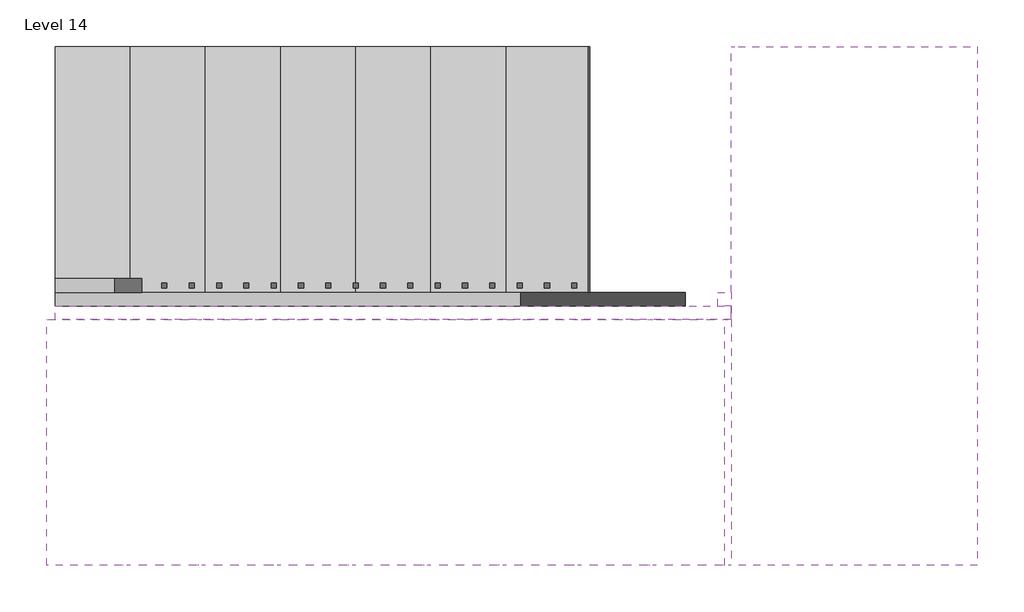
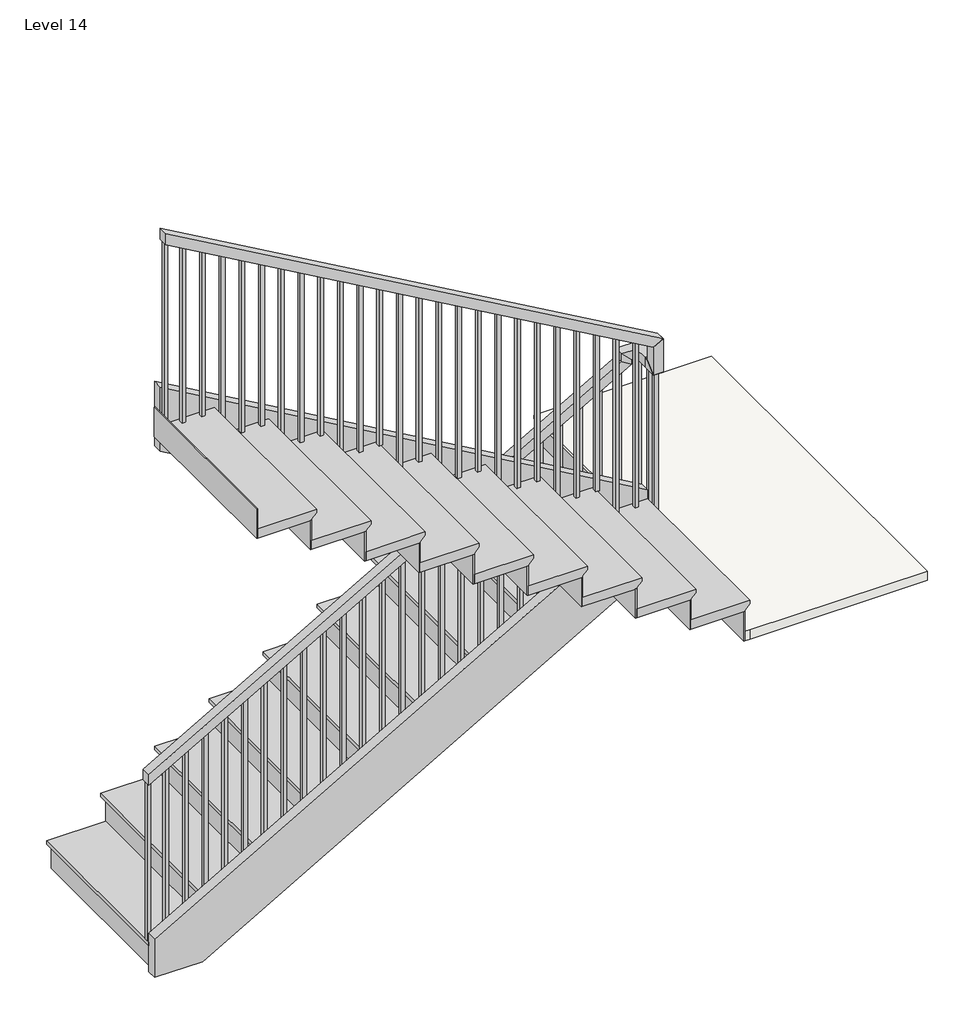
# One storey: 3 members, 2 stair flights, 1 railing, 1 slab.
"""IFC4 building model written with IfcOpenShell, lengths in millimetres."""

from ifc_helpers import new_model, si_unit, frame, origin, place, context, project, spatial, polyline, outline, extrude, faceted_brep, transform, mapped, element, save
from components import non_monolithic_landing_f7b8efd9, stair_flight_4ab4d81b, stair_flight_a571a0bd

model = new_model("IFC4")

# Units and contexts
model_context = context("Model", 3, world=origin())
ifc_project = project(units=[si_unit("LENGTHUNIT", "METRE", prefix="MILLI")], contexts=[model_context])

# Site, building, storey
site = spatial("IfcSite", under=ifc_project)
building = spatial("IfcBuilding", under=site)
storey = spatial("IfcBuildingStorey", under=building, Name="Level 14", Elevation=6400.8)

# Members
placement = place(None, origin())
element("IfcMember", 1, ObjectType="Stringer - 2\" Width", at=placement, inside=storey, context=model_context, shape_type="SweptSolid", body=[
    extrude(outline(polyline([(6609.8890626, -1591.1154463), (6400.8, -1591.1154463), (6400.8, -1342.8974141), (7669.724218, 872.6845537), (8020.9745172, 872.6845537), (6609.8890626, -1591.1154463)])), frame((0.0, -4788.1544725, 0.0), z_axis=(0.0, 1.0, 0.0), x_axis=(0.0, 0.0, 1.0)), (0.0, 0.0, 1.0), 50.8),
])
element("IfcMember", 2, ObjectType="Stringer - 2\" Width", at=placement, inside=storey, context=model_context, shape_type="SweptSolid", body=[
    extrude(outline(polyline([(7858.8387634, 923.4845537), (8210.0890626, 923.4845537), (9650.2690626, -1591.1154463), (9299.0187634, -1591.1154463), (7858.8387634, 923.4845537)])), frame((0.0, -4838.9544725, 0.0), z_axis=(0.0, 1.0, 0.0), x_axis=(0.0, 0.0, 1.0)), (0.0, 0.0, 1.0), 50.8),
])
element("IfcMember", 3, ObjectType="Stringer - 2\" Width", at=placement, inside=storey, context=model_context, shape_type="SweptSolid", body=[
    extrude(outline(polyline([(872.6845537, -4737.3544725), (923.4845537, -4737.3544725), (923.4845537, -4788.1544725), (872.6845537, -4788.1544725), (872.6845537, -4737.3544725)])), frame((0.0, 0.0, 7772.4), z_axis=(0.0, 0.0, 1.0), x_axis=(1.0, 0.0, 0.0)), (0.0, 0.0, 1.0), 304.8),
])

# Railing
element("IfcRailing", 4, ObjectType="Handrail - Rectangular", at=placement, inside=storey, context=model_context, shape_type="SolidModel", body=[
    faceted_brep([(-1591.1154463, -4686.5544725, 7475.22), (-1591.1154463, -4686.5544725, 7416.6782835), (-1591.1154463, -4737.3544725, 7416.6782835), (-1591.1154463, -4737.3544725, 7475.22), (847.2845537, -4686.5544725, 8871.7581818), (898.0845537, -4686.5544725, 8842.3110107), (898.0845537, -4737.3544725, 8842.3110107), (847.2845537, -4737.3544725, 8871.7581818), (847.2845537, -4686.5544725, 8915.4), (898.0845537, -4686.5544725, 8864.6), (898.0845537, -4737.3544725, 8864.6), (847.2845537, -4737.3544725, 8915.4), (974.2845537, -4686.5544725, 8915.4), (974.2845537, -4686.5544725, 8864.6), (923.4845537, -4737.3544725, 8864.6), (923.4845537, -4737.3544725, 8915.4), (974.2845537, -4813.5544725, 8915.4), (974.2845537, -4813.5544725, 8864.6), (923.4845537, -4813.5544725, 8864.6), (923.4845537, -4813.5544725, 8915.4), (974.2845537, -4838.9544725, 8915.4), (923.4845537, -4838.9544725, 8915.4), (923.4845537, -4889.7544725, 8864.6), (974.2845537, -4889.7544725, 8864.6)], [[[0, 1, 2, 3]], [[1, 0, 4, 5]], [[2, 1, 5, 6]], [[3, 2, 6, 7]], [[0, 3, 7, 4]], [[5, 4, 8, 9]], [[6, 5, 9, 10]], [[7, 6, 10, 11]], [[4, 7, 11, 8]], [[9, 8, 12, 13]], [[10, 9, 13, 14]], [[11, 10, 14, 15]], [[8, 11, 15, 12]], [[13, 12, 16, 17]], [[14, 13, 17, 18]], [[15, 14, 18, 19]], [[12, 15, 19, 16]], [[20, 21, 22, 23]], [[17, 16, 20, 23]], [[18, 17, 23, 22]], [[19, 18, 22, 21]], [[16, 19, 21, 20]]]),
    faceted_brep([(974.2845537, -4838.9544725, 8915.4), (974.2845537, -4889.7544725, 8864.6), (923.4845537, -4889.7544725, 8864.6), (923.4845537, -4838.9544725, 8915.4), (974.2845537, -4838.9544725, 9046.3254545), (923.4845537, -4838.9544725, 9016.8782835), (923.4845537, -4889.7544725, 9016.8782835), (974.2845537, -4889.7544725, 9046.3254545)], [[[0, 1, 2, 3]], [[4, 5, 6, 7]], [[1, 0, 4, 7]], [[2, 1, 7, 6]], [[3, 2, 6, 5]], [[0, 3, 5, 4]]]),
    faceted_brep([(974.2845537, -4889.7544725, 9046.3254545), (923.4845537, -4889.7544725, 9016.8782835), (923.4845537, -4838.9544725, 9016.8782835), (974.2845537, -4838.9544725, 9046.3254545), (-1591.1154463, -4889.7544725, 10515.6), (-1591.1154463, -4838.9544725, 10515.6), (-1591.1154463, -4838.9544725, 10457.0582835), (-1591.1154463, -4889.7544725, 10457.0582835)], [[[0, 1, 2, 3]], [[4, 5, 6, 7]], [[1, 0, 4, 7]], [[2, 1, 7, 6]], [[3, 2, 6, 5]], [[0, 3, 5, 4]]]),
    extrude(outline(polyline([(10393.4139653, -1479.9904463), (10404.3244198, -1499.0404463), (9441.18, -1499.0404463), (9441.18, -1479.9904463), (10393.4139653, -1479.9904463)])), frame((0.0, -4873.8794725, 0.0), z_axis=(0.0, 1.0, 0.0), x_axis=(0.0, 0.0, 1.0)), (0.0, 0.0, 1.0), 19.05),
    extrude(outline(polyline([(10335.2248744, -1378.3904463), (10346.1353289, -1397.4404463), (9441.18, -1397.4404463), (9441.18, -1378.3904463), (10335.2248744, -1378.3904463)])), frame((0.0, -4873.8794725, 0.0), z_axis=(0.0, 1.0, 0.0), x_axis=(0.0, 0.0, 1.0)), (0.0, 0.0, 1.0), 19.05),
    extrude(outline(polyline([(10277.0357835, -1276.7904463), (10287.946238, -1295.8404463), (9281.16, -1295.8404463), (9281.16, -1276.7904463), (10277.0357835, -1276.7904463)])), frame((0.0, -4873.8794725, 0.0), z_axis=(0.0, 1.0, 0.0), x_axis=(0.0, 0.0, 1.0)), (0.0, 0.0, 1.0), 19.05),
    extrude(outline(polyline([(10218.8466926, -1175.1904463), (10229.7571471, -1194.2404463), (9281.16, -1194.2404463), (9281.16, -1175.1904463), (10218.8466926, -1175.1904463)])), frame((0.0, -4873.8794725, 0.0), z_axis=(0.0, 1.0, 0.0), x_axis=(0.0, 0.0, 1.0)), (0.0, 0.0, 1.0), 19.05),
    extrude(outline(polyline([(10160.6576016, -1073.5904463), (10171.5680562, -1092.6404463), (9281.16, -1092.6404463), (9281.16, -1073.5904463), (10160.6576016, -1073.5904463)])), frame((0.0, -4873.8794725, 0.0), z_axis=(0.0, 1.0, 0.0), x_axis=(0.0, 0.0, 1.0)), (0.0, 0.0, 1.0), 19.05),
    extrude(outline(polyline([(10102.4685107, -971.9904463), (10113.3789653, -991.0404463), (9121.14, -991.0404463), (9121.14, -971.9904463), (10102.4685107, -971.9904463)])), frame((0.0, -4873.8794725, 0.0), z_axis=(0.0, 1.0, 0.0), x_axis=(0.0, 0.0, 1.0)), (0.0, 0.0, 1.0), 19.05),
    extrude(outline(polyline([(10044.2794198, -870.3904463), (10055.1898744, -889.4404463), (9121.14, -889.4404463), (9121.14, -870.3904463), (10044.2794198, -870.3904463)])), frame((0.0, -4873.8794725, 0.0), z_axis=(0.0, 1.0, 0.0), x_axis=(0.0, 0.0, 1.0)), (0.0, 0.0, 1.0), 19.05),
    extrude(outline(polyline([(9986.0903289, -768.7904463), (9997.0007835, -787.8404463), (9121.14, -787.8404463), (9121.14, -768.7904463), (9986.0903289, -768.7904463)])), frame((0.0, -4873.8794725, 0.0), z_axis=(0.0, 1.0, 0.0), x_axis=(0.0, 0.0, 1.0)), (0.0, 0.0, 1.0), 19.05),
    extrude(outline(polyline([(9927.901238, -667.1904463), (9938.8116926, -686.2404463), (8961.12, -686.2404463), (8961.12, -667.1904463), (9927.901238, -667.1904463)])), frame((0.0, -4873.8794725, 0.0), z_axis=(0.0, 1.0, 0.0), x_axis=(0.0, 0.0, 1.0)), (0.0, 0.0, 1.0), 19.05),
    extrude(outline(polyline([(9869.7121471, -565.5904463), (9880.6226016, -584.6404463), (8961.12, -584.6404463), (8961.12, -565.5904463), (9869.7121471, -565.5904463)])), frame((0.0, -4873.8794725, 0.0), z_axis=(0.0, 1.0, 0.0), x_axis=(0.0, 0.0, 1.0)), (0.0, 0.0, 1.0), 19.05),
    extrude(outline(polyline([(9811.5230562, -463.9904463), (9822.4335107, -483.0404463), (8961.12, -483.0404463), (8961.12, -463.9904463), (9811.5230562, -463.9904463)])), frame((0.0, -4873.8794725, 0.0), z_axis=(0.0, 1.0, 0.0), x_axis=(0.0, 0.0, 1.0)), (0.0, 0.0, 1.0), 19.05),
    extrude(outline(polyline([(9753.3339653, -362.3904463), (9764.2444198, -381.4404463), (8801.1, -381.4404463), (8801.1, -362.3904463), (9753.3339653, -362.3904463)])), frame((0.0, -4873.8794725, 0.0), z_axis=(0.0, 1.0, 0.0), x_axis=(0.0, 0.0, 1.0)), (0.0, 0.0, 1.0), 19.05),
    extrude(outline(polyline([(9695.1448744, -260.7904463), (9706.0553289, -279.8404463), (8801.1, -279.8404463), (8801.1, -260.7904463), (9695.1448744, -260.7904463)])), frame((0.0, -4873.8794725, 0.0), z_axis=(0.0, 1.0, 0.0), x_axis=(0.0, 0.0, 1.0)), (0.0, 0.0, 1.0), 19.05),
    extrude(outline(polyline([(9636.9557835, -159.1904463), (9647.866238, -178.2404463), (8641.08, -178.2404463), (8641.08, -159.1904463), (9636.9557835, -159.1904463)])), frame((0.0, -4873.8794725, 0.0), z_axis=(0.0, 1.0, 0.0), x_axis=(0.0, 0.0, 1.0)), (0.0, 0.0, 1.0), 19.05),
    extrude(outline(polyline([(9578.7666926, -57.5904463), (9589.6771471, -76.6404463), (8641.08, -76.6404463), (8641.08, -57.5904463), (9578.7666926, -57.5904463)])), frame((0.0, -4873.8794725, 0.0), z_axis=(0.0, 1.0, 0.0), x_axis=(0.0, 0.0, 1.0)), (0.0, 0.0, 1.0), 19.05),
    extrude(outline(polyline([(9520.5776016, 44.0095537), (9531.4880562, 24.9595537), (8641.08, 24.9595537), (8641.08, 44.0095537), (9520.5776016, 44.0095537)])), frame((0.0, -4873.8794725, 0.0), z_axis=(0.0, 1.0, 0.0), x_axis=(0.0, 0.0, 1.0)), (0.0, 0.0, 1.0), 19.05),
    extrude(outline(polyline([(9462.3885107, 145.6095537), (9473.2989653, 126.5595537), (8481.06, 126.5595537), (8481.06, 145.6095537), (9462.3885107, 145.6095537)])), frame((0.0, -4873.8794725, 0.0), z_axis=(0.0, 1.0, 0.0), x_axis=(0.0, 0.0, 1.0)), (0.0, 0.0, 1.0), 19.05),
    extrude(outline(polyline([(9404.1994198, 247.2095537), (9415.1098744, 228.1595537), (8481.06, 228.1595537), (8481.06, 247.2095537), (9404.1994198, 247.2095537)])), frame((0.0, -4873.8794725, 0.0), z_axis=(0.0, 1.0, 0.0), x_axis=(0.0, 0.0, 1.0)), (0.0, 0.0, 1.0), 19.05),
    extrude(outline(polyline([(9346.0103289, 348.8095537), (9356.9207835, 329.7595537), (8481.06, 329.7595537), (8481.06, 348.8095537), (9346.0103289, 348.8095537)])), frame((0.0, -4873.8794725, 0.0), z_axis=(0.0, 1.0, 0.0), x_axis=(0.0, 0.0, 1.0)), (0.0, 0.0, 1.0), 19.05),
    extrude(outline(polyline([(9287.821238, 450.4095537), (9298.7316926, 431.3595537), (8321.04, 431.3595537), (8321.04, 450.4095537), (9287.821238, 450.4095537)])), frame((0.0, -4873.8794725, 0.0), z_axis=(0.0, 1.0, 0.0), x_axis=(0.0, 0.0, 1.0)), (0.0, 0.0, 1.0), 19.05),
    extrude(outline(polyline([(9229.6321471, 552.0095537), (9240.5426016, 532.9595537), (8321.04, 532.9595537), (8321.04, 552.0095537), (9229.6321471, 552.0095537)])), frame((0.0, -4873.8794725, 0.0), z_axis=(0.0, 1.0, 0.0), x_axis=(0.0, 0.0, 1.0)), (0.0, 0.0, 1.0), 19.05),
    extrude(outline(polyline([(9171.4430562, 653.6095537), (9182.3535107, 634.5595537), (8321.04, 634.5595537), (8321.04, 653.6095537), (9171.4430562, 653.6095537)])), frame((0.0, -4873.8794725, 0.0), z_axis=(0.0, 1.0, 0.0), x_axis=(0.0, 0.0, 1.0)), (0.0, 0.0, 1.0), 19.05),
    extrude(outline(polyline([(9113.2539653, 755.2095537), (9124.1644198, 736.1595537), (8161.02, 736.1595537), (8161.02, 755.2095537), (9113.2539653, 755.2095537)])), frame((0.0, -4873.8794725, 0.0), z_axis=(0.0, 1.0, 0.0), x_axis=(0.0, 0.0, 1.0)), (0.0, 0.0, 1.0), 19.05),
    extrude(outline(polyline([(9055.0648744, 856.8095537), (9065.9753289, 837.7595537), (8161.02, 837.7595537), (8161.02, 856.8095537), (9055.0648744, 856.8095537)])), frame((0.0, -4873.8794725, 0.0), z_axis=(0.0, 1.0, 0.0), x_axis=(0.0, 0.0, 1.0)), (0.0, 0.0, 1.0), 19.05),
    extrude(outline(polyline([(939.3595537, -4804.0294725), (958.4095537, -4804.0294725), (958.4095537, -4823.0794725), (939.3595537, -4823.0794725), (939.3595537, -4804.0294725)])), frame((0.0, 0.0, 8001.0), z_axis=(0.0, 0.0, 1.0), x_axis=(1.0, 0.0, 0.0)), (0.0, 0.0, 1.0), 863.6),
    extrude(outline(polyline([(8818.6716926, 856.8095537), (8807.761238, 837.7595537), (7840.98, 837.7595537), (7840.98, 856.8095537), (8818.6716926, 856.8095537)])), frame((0.0, -4721.4794725, 0.0), z_axis=(0.0, 1.0, 0.0), x_axis=(0.0, 0.0, 1.0)), (0.0, 0.0, 1.0), 19.05),
    extrude(outline(polyline([(8760.4826016, 755.2095537), (8749.5721471, 736.1595537), (7840.98, 736.1595537), (7840.98, 755.2095537), (8760.4826016, 755.2095537)])), frame((0.0, -4721.4794725, 0.0), z_axis=(0.0, 1.0, 0.0), x_axis=(0.0, 0.0, 1.0)), (0.0, 0.0, 1.0), 19.05),
    extrude(outline(polyline([(8702.2935107, 653.6095537), (8691.3830562, 634.5595537), (7840.98, 634.5595537), (7840.98, 653.6095537), (8702.2935107, 653.6095537)])), frame((0.0, -4721.4794725, 0.0), z_axis=(0.0, 1.0, 0.0), x_axis=(0.0, 0.0, 1.0)), (0.0, 0.0, 1.0), 19.05),
    extrude(outline(polyline([(8644.1044198, 552.0095537), (8633.1939653, 532.9595537), (7680.96, 532.9595537), (7680.96, 552.0095537), (8644.1044198, 552.0095537)])), frame((0.0, -4721.4794725, 0.0), z_axis=(0.0, 1.0, 0.0), x_axis=(0.0, 0.0, 1.0)), (0.0, 0.0, 1.0), 19.05),
    extrude(outline(polyline([(8585.9153289, 450.4095537), (8575.0048744, 431.3595537), (7680.96, 431.3595537), (7680.96, 450.4095537), (8585.9153289, 450.4095537)])), frame((0.0, -4721.4794725, 0.0), z_axis=(0.0, 1.0, 0.0), x_axis=(0.0, 0.0, 1.0)), (0.0, 0.0, 1.0), 19.05),
    extrude(outline(polyline([(8527.726238, 348.8095537), (8516.8157835, 329.7595537), (7520.94, 329.7595537), (7520.94, 348.8095537), (8527.726238, 348.8095537)])), frame((0.0, -4721.4794725, 0.0), z_axis=(0.0, 1.0, 0.0), x_axis=(0.0, 0.0, 1.0)), (0.0, 0.0, 1.0), 19.05),
    extrude(outline(polyline([(8469.5371471, 247.2095537), (8458.6266926, 228.1595537), (7520.94, 228.1595537), (7520.94, 247.2095537), (8469.5371471, 247.2095537)])), frame((0.0, -4721.4794725, 0.0), z_axis=(0.0, 1.0, 0.0), x_axis=(0.0, 0.0, 1.0)), (0.0, 0.0, 1.0), 19.05),
    extrude(outline(polyline([(8411.3480562, 145.6095537), (8400.4376016, 126.5595537), (7520.94, 126.5595537), (7520.94, 145.6095537), (8411.3480562, 145.6095537)])), frame((0.0, -4721.4794725, 0.0), z_axis=(0.0, 1.0, 0.0), x_axis=(0.0, 0.0, 1.0)), (0.0, 0.0, 1.0), 19.05),
    extrude(outline(polyline([(8353.1589653, 44.0095537), (8342.2485107, 24.9595537), (7360.92, 24.9595537), (7360.92, 44.0095537), (8353.1589653, 44.0095537)])), frame((0.0, -4721.4794725, 0.0), z_axis=(0.0, 1.0, 0.0), x_axis=(0.0, 0.0, 1.0)), (0.0, 0.0, 1.0), 19.05),
    extrude(outline(polyline([(8294.9698744, -57.5904463), (8284.0594198, -76.6404463), (7360.92, -76.6404463), (7360.92, -57.5904463), (8294.9698744, -57.5904463)])), frame((0.0, -4721.4794725, 0.0), z_axis=(0.0, 1.0, 0.0), x_axis=(0.0, 0.0, 1.0)), (0.0, 0.0, 1.0), 19.05),
    extrude(outline(polyline([(8236.7807835, -159.1904463), (8225.8703289, -178.2404463), (7360.92, -178.2404463), (7360.92, -159.1904463), (8236.7807835, -159.1904463)])), frame((0.0, -4721.4794725, 0.0), z_axis=(0.0, 1.0, 0.0), x_axis=(0.0, 0.0, 1.0)), (0.0, 0.0, 1.0), 19.05),
    extrude(outline(polyline([(8178.5916926, -260.7904463), (8167.681238, -279.8404463), (7200.9, -279.8404463), (7200.9, -260.7904463), (8178.5916926, -260.7904463)])), frame((0.0, -4721.4794725, 0.0), z_axis=(0.0, 1.0, 0.0), x_axis=(0.0, 0.0, 1.0)), (0.0, 0.0, 1.0), 19.05),
    extrude(outline(polyline([(8120.4026016, -362.3904463), (8109.4921471, -381.4404463), (7200.9, -381.4404463), (7200.9, -362.3904463), (8120.4026016, -362.3904463)])), frame((0.0, -4721.4794725, 0.0), z_axis=(0.0, 1.0, 0.0), x_axis=(0.0, 0.0, 1.0)), (0.0, 0.0, 1.0), 19.05),
    extrude(outline(polyline([(8062.2135107, -463.9904463), (8051.3030562, -483.0404463), (7200.9, -483.0404463), (7200.9, -463.9904463), (8062.2135107, -463.9904463)])), frame((0.0, -4721.4794725, 0.0), z_axis=(0.0, 1.0, 0.0), x_axis=(0.0, 0.0, 1.0)), (0.0, 0.0, 1.0), 19.05),
    extrude(outline(polyline([(8004.0244198, -565.5904463), (7993.1139653, -584.6404463), (7040.88, -584.6404463), (7040.88, -565.5904463), (8004.0244198, -565.5904463)])), frame((0.0, -4721.4794725, 0.0), z_axis=(0.0, 1.0, 0.0), x_axis=(0.0, 0.0, 1.0)), (0.0, 0.0, 1.0), 19.05),
    extrude(outline(polyline([(7945.8353289, -667.1904463), (7934.9248744, -686.2404463), (7040.88, -686.2404463), (7040.88, -667.1904463), (7945.8353289, -667.1904463)])), frame((0.0, -4721.4794725, 0.0), z_axis=(0.0, 1.0, 0.0), x_axis=(0.0, 0.0, 1.0)), (0.0, 0.0, 1.0), 19.05),
    extrude(outline(polyline([(7887.646238, -768.7904463), (7876.7357835, -787.8404463), (6880.86, -787.8404463), (6880.86, -768.7904463), (7887.646238, -768.7904463)])), frame((0.0, -4721.4794725, 0.0), z_axis=(0.0, 1.0, 0.0), x_axis=(0.0, 0.0, 1.0)), (0.0, 0.0, 1.0), 19.05),
    extrude(outline(polyline([(7829.4571471, -870.3904463), (7818.5466926, -889.4404463), (6880.86, -889.4404463), (6880.86, -870.3904463), (7829.4571471, -870.3904463)])), frame((0.0, -4721.4794725, 0.0), z_axis=(0.0, 1.0, 0.0), x_axis=(0.0, 0.0, 1.0)), (0.0, 0.0, 1.0), 19.05),
    extrude(outline(polyline([(7771.2680562, -971.9904463), (7760.3576016, -991.0404463), (6880.86, -991.0404463), (6880.86, -971.9904463), (7771.2680562, -971.9904463)])), frame((0.0, -4721.4794725, 0.0), z_axis=(0.0, 1.0, 0.0), x_axis=(0.0, 0.0, 1.0)), (0.0, 0.0, 1.0), 19.05),
    extrude(outline(polyline([(7713.0789653, -1073.5904463), (7702.1685107, -1092.6404463), (6720.84, -1092.6404463), (6720.84, -1073.5904463), (7713.0789653, -1073.5904463)])), frame((0.0, -4721.4794725, 0.0), z_axis=(0.0, 1.0, 0.0), x_axis=(0.0, 0.0, 1.0)), (0.0, 0.0, 1.0), 19.05),
    extrude(outline(polyline([(7654.8898744, -1175.1904463), (7643.9794198, -1194.2404463), (6720.84, -1194.2404463), (6720.84, -1175.1904463), (7654.8898744, -1175.1904463)])), frame((0.0, -4721.4794725, 0.0), z_axis=(0.0, 1.0, 0.0), x_axis=(0.0, 0.0, 1.0)), (0.0, 0.0, 1.0), 19.05),
    extrude(outline(polyline([(7596.7007835, -1276.7904463), (7585.7903289, -1295.8404463), (6720.84, -1295.8404463), (6720.84, -1276.7904463), (7596.7007835, -1276.7904463)])), frame((0.0, -4721.4794725, 0.0), z_axis=(0.0, 1.0, 0.0), x_axis=(0.0, 0.0, 1.0)), (0.0, 0.0, 1.0), 19.05),
    extrude(outline(polyline([(7538.5116926, -1378.3904463), (7527.601238, -1397.4404463), (6560.82, -1397.4404463), (6560.82, -1378.3904463), (7538.5116926, -1378.3904463)])), frame((0.0, -4721.4794725, 0.0), z_axis=(0.0, 1.0, 0.0), x_axis=(0.0, 0.0, 1.0)), (0.0, 0.0, 1.0), 19.05),
    extrude(outline(polyline([(7480.3226016, -1479.9904463), (7469.4121471, -1499.0404463), (6560.82, -1499.0404463), (6560.82, -1479.9904463), (7480.3226016, -1479.9904463)])), frame((0.0, -4721.4794725, 0.0), z_axis=(0.0, 1.0, 0.0), x_axis=(0.0, 0.0, 1.0)), (0.0, 0.0, 1.0), 19.05),
    extrude(outline(polyline([(939.3595537, -4854.8294725), (958.4095537, -4854.8294725), (958.4095537, -4873.8794725), (939.3595537, -4873.8794725), (939.3595537, -4854.8294725)])), frame((0.0, 0.0, 8001.0), z_axis=(0.0, 0.0, 1.0), x_axis=(1.0, 0.0, 0.0)), (0.0, 0.0, 1.0), 863.6),
    extrude(outline(polyline([(939.3595537, -4721.4794725), (939.3595537, -4702.4294725), (958.4095537, -4702.4294725), (958.4095537, -4721.4794725), (939.3595537, -4721.4794725)])), frame((0.0, 0.0, 8001.0), z_axis=(0.0, 0.0, 1.0), x_axis=(1.0, 0.0, 0.0)), (0.0, 0.0, 1.0), 863.6),
    extrude(outline(polyline([(10446.1478289, -1572.0654463), (10457.0582835, -1591.1154463), (9441.18, -1591.1154463), (9441.18, -1572.0654463), (10446.1478289, -1572.0654463)])), frame((0.0, -4873.8794725, 0.0), z_axis=(0.0, 1.0, 0.0), x_axis=(0.0, 0.0, 1.0)), (0.0, 0.0, 1.0), 19.05),
    extrude(outline(polyline([(7427.588738, -1572.0654463), (7416.6782835, -1591.1154463), (6560.82, -1591.1154463), (6560.82, -1572.0654463), (7427.588738, -1572.0654463)])), frame((0.0, -4721.4794725, 0.0), z_axis=(0.0, 1.0, 0.0), x_axis=(0.0, 0.0, 1.0)), (0.0, 0.0, 1.0), 19.05),
])

# Slab
non_monolithic_landing_shape = non_monolithic_landing_f7b8efd9(model_context)
element("IfcSlab", 5, ObjectType="Non-Monolithic Landing", at=placement, inside=storey, context=model_context, shape_type="MappedRepresentation", body=[
    mapped(non_monolithic_landing_shape, transform((0.0, 0.0, 0.0), x_axis=(1.0, 0.0, 0.0), y_axis=(0.0, 1.0, 0.0), z_axis=(0.0, 0.0, 1.0))),
])

# Stair flights
stair_flight_shape = stair_flight_4ab4d81b(model_context)
element("IfcStairFlight", 6, ObjectType="2\" Tread 1\" Nosing 1/4\" Riser", at=placement, inside=storey, context=model_context, shape_type="MappedRepresentation", body=[
    mapped(stair_flight_shape, transform((0.0, 0.0, 0.0), x_axis=(1.0, 0.0, 0.0), y_axis=(0.0, 1.0, 0.0), z_axis=(0.0, 0.0, 1.0))),
])
stair_flight_2_shape = stair_flight_a571a0bd(model_context)
element("IfcStairFlight", 7, ObjectType="2\" Tread 1\" Nosing 1/4\" Riser", at=placement, inside=storey, context=model_context, shape_type="MappedRepresentation", body=[
    mapped(stair_flight_2_shape, transform((0.0, 0.0, 0.0), x_axis=(1.0, 0.0, 0.0), y_axis=(0.0, 1.0, 0.0), z_axis=(0.0, 0.0, 1.0))),
])

save(model, "model.ifc")

# Revit data of these elements
# Type "Handrail - Rectangular"
#   Assembly Code = "C2010400"
#   built-in parameter 1008612 = 0.0416667 (stored number, unit not read)
#   built-in parameter 1008611 = 0.0416667 (stored number, unit not read)
#   built-in parameter 1008609 = 0.333333 (stored number, unit not read)
#   built-in parameter 1008604 = 0.166667 (stored number, unit not read)
#   built-in parameter 1008603 = 0.166667 (stored number, unit not read)
#   Railing Height = 3' - 0"
#   built-in parameter 1008630 = 2
#   built-in parameter 1008610 = 2
#   built-in parameter 1008618 = Baluster - Square : 3/4"
# Elements 1, 2, 3 (IfcMember, "Stringer - 2\" Width")
#   Phase Created = New Construction
# Element 4 (IfcRailing, "Handrail - Rectangular")
#   Phase Created = New Construction
# Element 5 (IfcSlab, "Non-Monolithic Landing")
#   Phase Created = New Construction
# Elements 6, 7 (IfcStairFlight, "2\" Tread 1\" Nosing 1/4\" Riser")
#   Phase Created = New Construction
